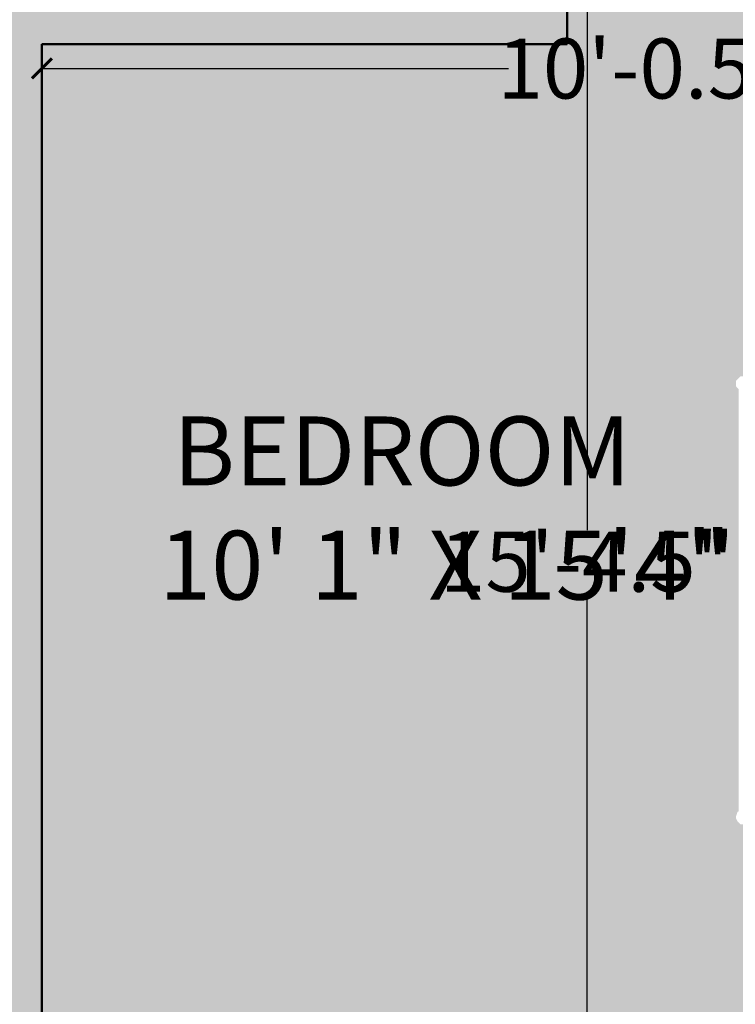
# Model space of a CAD drawing. Units: inches. Extents: x 528 to 2620, y -1066 to 798.
# Tile 12 of 41: x 776 to 848, y 573 to 672. Entities that reach past the tile are written whole.
import ezdxf

# ---------------------------------------------------------------- set-up
doc = ezdxf.new("R2010")
doc.units = ezdxf.units.IN
doc.header["$MEASUREMENT"] = 0
for name, color, linetype, lineweight in [('A-ANNO-DIMS', 2, 'Continuous', 18), ('A-AREA-IDEN', 7, 'Continuous', 18), ('A-WALL', 7, 'Continuous', 50), ('A-WALL-PATT', 8, 'Continuous', 13)]:
    doc.layers.add(name, color=color, linetype=linetype, lineweight=lineweight)
doc.styles.get("Standard").update_dxf_attribs({"font": 'arial.ttf'})
doc.dimstyles.get("Standard").update_dxf_attribs({"dimtxt": 6, "dimasz": 2, "dimexe": 0.18, "dimexo": 0.0625, "dimgap": 0.09, "dimtad": 0, "dimtih": 1, "dimtoh": 1, "dimdec": 1, "dimzin": 0, "dimdsep": 46, "dimlunit": 3, "dimtxsty": 'Standard', "dimblk": 'ARCHTICK', "dimcen": 0.09, "dimadec": 0, "dimazin": 0, "dimtfac": 1, "dimtdec": 1, "dimtofl": 0, "dimtmove": 0, "dimatfit": 3, "dimfxl": 1, "dimtolj": 1, "dimtzin": 0, "dimarcsym": 0})

# ---------------------------------------------------------------- blocks, each defined once
blk = doc.blocks.new('_ArchTick')
at = {"color": 0, "linetype": 'ByBlock', "const_width": 0.15}
blk.add_lwpolyline([(-0.5, -0.5), (0.5, 0.5)], dxfattribs=at)
blk = doc.blocks.new('*D27')
at = {"layer": 'A-ANNO-DIMS', "color": 0, "lineweight": -2, "transparency": 16777216}
for p, q in [((778.559, 667.76), (778.559, 666.811)), ((899.059, 667.76), (899.059, 666.811)), ((778.559, 666.991), (825.201, 666.991)), ((899.059, 666.991), (852.418, 666.991))]:
    blk.add_line(p, q, dxfattribs=at)
at = {"layer": 'Defpoints', "color": 0, "transparency": 16777216}
for p in [(778.559, 667.823), (899.059, 667.823), (899.059, 666.991)]:
    blk.add_point(p, dxfattribs=at)
at = {"layer": 'A-ANNO-DIMS', "color": 0, "lineweight": -2, "transparency": 16777216, "xscale": 2, "yscale": 2, "zscale": 2, "rotation": 180}
blk.add_blockref('_ArchTick', (778.559, 666.991), dxfattribs=at)
at = {"layer": 'A-ANNO-DIMS', "color": 0, "lineweight": -2, "transparency": 16777216, "xscale": 2, "yscale": 2, "zscale": 2}
blk.add_blockref('_ArchTick', (899.059, 666.991), dxfattribs=at)
at = {"layer": 'A-ANNO-DIMS', "color": 0, "transparency": 16777216, "insert": (838.809, 666.991), "char_height": 6, "attachment_point": 5}
blk.add_mtext('\\A1;10\'-0.5"', dxfattribs=at)
blk = doc.blocks.new('*D28')
at = {"layer": 'A-ANNO-DIMS', "color": 0, "lineweight": -2, "transparency": 16777216}
for p, q in [((833.059, 709.922), (833.059, 620.826)), ((833.122, 709.922), (833.239, 709.922)), ((833.059, 525.422), (833.059, 614.519)), ((833.102, 525.422), (832.879, 525.422))]:
    blk.add_line(p, q, dxfattribs=at)
at = {"layer": 'Defpoints', "color": 0, "transparency": 16777216}
for p in [(833.059, 709.922), (833.059, 709.922), (833.164, 525.422)]:
    blk.add_point(p, dxfattribs=at)
at = {"layer": 'A-ANNO-DIMS', "color": 0, "lineweight": -2, "transparency": 16777216, "xscale": 2, "yscale": 2, "zscale": 2}
for p, rotation in [((833.059, 709.922), 90), ((833.059, 525.422), 270)]:
    blk.add_blockref('_ArchTick', p, dxfattribs=dict(at, rotation=rotation))
at = {"layer": 'A-ANNO-DIMS', "color": 0, "transparency": 16777216, "insert": (833.059, 617.672), "char_height": 6, "attachment_point": 5}
blk.add_mtext('\\A1;15\'-4.5"', dxfattribs=at)

msp = doc.modelspace()

# ---------------------------------------------------------------- hatches: boundary and pattern name
at = {"layer": 'A-WALL-PATT', "transparency": 33554687}
h = msp.add_hatch(color=256, dxfattribs=at)
h.dxf.hatch_style = 1
h.paths.add_polyline_path([(861.059, 273.922), (817.059, 273.922), (817.059, 272.922), (861.059, 272.922)])
h.paths.add_polyline_path([(817.059, 277.922), (815.059, 277.922), (815.059, 268.922), (817.059, 268.922)])
h.paths.add_polyline_path([(908.059, 397.922), (899.059, 397.922), (899.059, 395.922), (908.059, 395.922)])
h.paths.add_polyline_path([(908.059, 443.922), (899.059, 443.922), (899.059, 441.922), (908.059, 441.922)])
h.paths.add_polyline_path([(904.059, 441.922), (903.059, 441.922), (903.059, 397.922), (904.059, 397.922)])
h.paths.add_polyline_path([(625.059, 561.422), (624.059, 561.422), (624.059, 537.422), (625.059, 537.422)])
h.paths.add_polyline_path([(648.747, 334.444), (720.045, 334.444), (720.045, 344.998), (648.747, 344.998)], flags=9)
h.paths.add_polyline_path([(819.733, 323.153), (880.328, 323.153), (880.328, 333.708), (819.733, 333.708)], flags=9)
h.paths.add_polyline_path([(779.898, 680.607), (821.764, 680.607), (821.764, 691.169), (779.898, 691.169)], flags=9)
h.paths.add_polyline_path([(779.876, 692.362), (817.138, 692.362), (817.138, 703.058), (779.876, 703.058)], flags=9)
h.paths.add_polyline_path([(799.994, 453.884), (860.589, 453.884), (860.589, 464.439), (799.994, 464.439)], flags=9)
h.paths.add_polyline_path([(650.866, 539.397), (708.781, 539.397), (708.781, 549.952), (650.866, 549.952)], flags=9)
h.paths.add_polyline_path([(788.504, 612.01), (849.099, 612.01), (849.099, 622.565), (788.504, 622.565)], flags=9)
h.paths.add_polyline_path([(639.539, 648.31), (700.134, 648.31), (700.134, 658.865), (639.539, 658.865)], flags=9)
h.paths.add_polyline_path([(648.913, 346.09), (747.706, 346.09), (747.706, 356.778), (648.913, 356.778)], flags=9)
h.paths.add_polyline_path([(676.857, 450.66), (746.735, 450.66), (746.735, 461.355), (676.857, 461.355)], flags=9)
h.paths.add_polyline_path([(819.711, 334.947), (865.526, 334.947), (865.526, 345.636), (819.711, 345.636)], flags=9)
h.paths.add_polyline_path([(806.298, 467.745), (874.047, 467.745), (874.047, 478.441), (806.298, 478.441)], flags=9)
h.paths.add_polyline_path([(653.235, 552.284), (690.497, 552.284), (690.497, 562.979), (653.235, 562.979)], flags=9)
h.paths.add_polyline_path([(789.903, 623.407), (843.208, 623.407), (843.208, 634.103), (789.903, 634.103)], flags=9)
h.paths.add_polyline_path([(639.773, 662.103), (693.077, 662.103), (693.077, 672.798), (639.773, 672.798)], flags=9)
h.paths.add_polyline_path([(801.587, 242.914), (846.334, 242.914), (846.334, 253.603), (801.587, 253.603)], flags=9)
h.paths.add_polyline_path([(925.362, 593.982), (925.362, 674.057), (914.673, 674.057), (914.673, 593.982)], flags=9)
h.paths.add_polyline_path([(612.559, 593.982), (612.559, 674.057), (601.871, 674.057), (601.871, 593.982)], flags=9)
h.paths.add_polyline_path([(723.31, 726.564), (803.385, 726.564), (803.385, 737.252), (723.31, 737.252)], flags=9)
at = {"layer": 'A-WALL-PATT', "transparency": 33554521}
h = msp.add_hatch(color=256, dxfattribs=at)
h.dxf.hatch_style = 1
h.paths.add_polyline_path([(629.059, 709.922), (677.559, 709.922), (677.559, 718.922), (620.059, 718.922), (620.059, 667.922), (629.059, 667.922)])
h.paths.add_polyline_path([(790.559, 718.922), (725.559, 718.922), (725.559, 709.922), (774.059, 709.922), (774.059, 577.922), (768.481, 577.922), (768.559, 573.422), (774.059, 573.422), (774.059, 567.422), (778.559, 567.422), (778.559, 669.422), (831.059, 669.422), (831.059, 675.922), (826.559, 675.922), (826.559, 673.922), (778.559, 673.922), (778.559, 709.922), (790.559, 709.922)])
h.paths.add_polyline_path([(908.059, 718.922), (879.059, 718.922), (879.059, 709.922), (899.059, 709.922), (899.059, 641.672), (908.059, 641.672)])
h.paths.add_polyline_path([(629.059, 619.922), (620.059, 619.922), (620.059, 561.422), (629.059, 561.422), (629.059, 573.422), (724.059, 573.422), (724.059, 569.422), (728.559, 569.422), (728.559, 577.922), (629.059, 577.922)])
h.paths.add_polyline_path([(779.059, 391.422), (779.059, 400.422), (770.059, 400.422), (764.059, 400.422), (764.059, 397.422), (764.059, 391.422), (770.059, 391.422), (770.059, 268.922), (815.059, 268.922), (815.059, 277.922), (779.059, 277.922), (779.059, 359.767)])
h.paths.add_polyline_path([(908.059, 395.922), (899.059, 395.922), (851.059, 395.922), (851.059, 391.422), (899.059, 391.422), (899.059, 277.922), (863.059, 277.922), (863.059, 268.922), (908.059, 268.922)])
h.paths.add_polyline_path([(908.059, 593.672), (899.059, 593.672), (899.059, 525.422), (778.559, 525.422), (778.559, 527.172), (774.059, 527.172), (774.059, 520.922), (899.059, 520.922), (899.059, 443.922), (908.059, 443.922)])
h.paths.add_polyline_path([(629.059, 520.922), (728.559, 520.922), (728.559, 545.422), (724.059, 545.422), (724.059, 525.422), (629.059, 525.422), (629.059, 537.422), (620.059, 537.422), (620.059, 484.672), (629.059, 484.672)])
h.paths.add_polyline_path([(629.059, 436.672), (620.059, 436.672), (620.059, 391.422), (648.559, 391.422), (648.559, 400.422), (629.059, 400.422)])
h.paths.add_polyline_path([(716.059, 397.422), (716.059, 400.422), (696.559, 400.422), (696.559, 391.422), (716.059, 391.422)])
at = {"layer": 'A-WALL-PATT', "transparency": 33554590}
h = msp.add_hatch(color=256, dxfattribs=at)
h.dxf.hatch_style = 1
h.paths.add_polyline_path([(774.059, 709.922), (629.059, 709.922), (629.059, 577.922), (728.559, 577.922), (728.559, 579.422), (728.559, 619.422), (730.309, 619.422), (730.309, 619.384, -0.401453), (768.559, 579.422), (768.559, 577.922), (774.059, 577.922)])
h.paths.add_polyline_path([(723.896, 686.058), (723.968, 686.064), (723.828, 686.128)], flags=0)
h.paths.add_polyline_path([(722.785, 642.699), (722.893, 642.756), (722.893, 684.992), (722.647, 685.244), (722.647, 685.82), (723.079, 686.262), (723.533, 686.262), (723.968, 686.064), (724.739, 686.128), (770.696, 686.128), (770.78, 686.14), (771.126, 686.266), (771.694, 686.094), (771.94, 685.478), (771.67, 684.904), (771.582, 684.871), (771.582, 642.782), (771.878, 642.514), (771.878, 641.921), (771.511, 641.462), (770.855, 641.462), (770.401, 641.833), (770.401, 641.551), (724.739, 641.551), (723.991, 641.705), (723.443, 641.414), (722.879, 641.585), (722.597, 642.142)], flags=16)
h.paths.add_polyline_path([(723.994, 641.704), (723.994, 641.707), (723.991, 641.705)], flags=0)
h.paths.add_polyline_path([(722.893, 642.732), (722.893, 684.992), (722.647, 685.244), (722.647, 685.82), (723.079, 686.262), (723.287, 686.262), (722.991, 686.172), (722.794, 685.971), (722.647, 685.68), (722.647, 685.434), (722.745, 685.143), (722.942, 684.942), (723.238, 684.807), (723.484, 684.807), (723.779, 684.897), (723.976, 685.098), (724.174, 685.488), (724.124, 685.635), (724.124, 685.249), (723.631, 684.746), (723.631, 642.961), (724.124, 642.514), (724.124, 641.887), (723.656, 641.462), (723.079, 641.462), (722.647, 641.904), (722.647, 642.48)], flags=0)
h.paths.add_polyline_path([(722.647, 642.29), (722.647, 642.044), (722.794, 641.753), (723.079, 641.462), (723.287, 641.462), (722.879, 641.585), (722.597, 642.142)], flags=0)
h.paths.add_polyline_path([(770.745, 686.128), (770.58, 686.128), (770.551, 686.057)], flags=0)
h.paths.add_polyline_path([(743.299, 645.288), (753.227, 659.398), (748.69, 663.75), (753.234, 668.538), (743.299, 682.458), (743.791, 682.592), (744.136, 682.681), (744.53, 682.928), (744.628, 683.084), (745.017, 683.327), (744.53, 684.069), (744.776, 684.158), (744.874, 684.315), (745.514, 684.404), (746.081, 684.651), (746.474, 684.651), (746.819, 684.807), (747.459, 685.031), (747.705, 685.143), (748.198, 685.277), (748.394, 685.523), (748.862, 685.523), (749.994, 686.128), (753.488, 676.03), (757.379, 680.153), (757.791, 679.758), (758.044, 680.645), (758.29, 681.227), (758.29, 682.055), (758.019, 682.592), (757.871, 683.174), (757.822, 683.778), (758.388, 684.069), (758.979, 684.203), (759.619, 684.158), (760.21, 683.957), (760.751, 683.666), (761.859, 683.666), (762.401, 683.957), (762.991, 684.114), (763.631, 684.114), (764.198, 683.957), (764.739, 683.666), (766.118, 683.666), (766.659, 683.957), (767.25, 684.158), (767.865, 684.203), (768.456, 684.069), (769.047, 683.778), (768.998, 683.174), (768.85, 682.592), (768.554, 682.055), (768.554, 681.227), (768.801, 680.645), (769.092, 679.75), (768.948, 678.832), (768.801, 678.228), (768.554, 677.646), (768.554, 676.818), (768.801, 676.237), (769.092, 675.341), (768.948, 674.424), (768.801, 673.82), (768.554, 673.283), (768.554, 672.41), (768.801, 671.873), (768.998, 671.291), (769.047, 670.642), (768.948, 670.016), (768.801, 669.411), (768.554, 668.874), (768.554, 668.002), (768.974, 667.239), (769.047, 666.279), (769.047, 665.563), (768.456, 665.316), (767.865, 665.16), (767.25, 665.16), (766.659, 665.361), (766.118, 665.697), (764.739, 665.697), (763.945, 665.204), (762.991, 665.204), (762.401, 665.361), (761.859, 665.697), (761.005, 665.697), (762.696, 664.086), (760.741, 662.027), (761.859, 662.027), (762.401, 662.318), (763.342, 662.548), (764.247, 662.318), (764.788, 662.027), (766.118, 662.027), (766.659, 662.318), (767.25, 662.519), (767.865, 662.564), (768.505, 662.43), (769.047, 662.116), (769.047, 661.4), (769.047, 660.796), (768.85, 660.214), (768.554, 659.677), (768.554, 658.849), (768.85, 658.267), (768.998, 657.663), (769.069, 656.749), (768.85, 655.851), (768.554, 655.269), (768.554, 654.441), (768.85, 653.859), (769.069, 652.961), (768.998, 652.046), (768.85, 651.442), (768.554, 650.905), (768.554, 650.032), (768.85, 649.495), (768.998, 648.914), (769.047, 648.265), (768.998, 647.638), (768.85, 647.034), (768.554, 646.497), (768.554, 645.624), (768.85, 645.087), (769.047, 644.55), (769.047, 643.901), (768.505, 643.655), (767.865, 643.521), (767.25, 643.521), (766.659, 643.722), (766.118, 644.058), (764.788, 644.058), (764.247, 643.722), (763.342, 643.492), (762.401, 643.722), (761.859, 644.058), (760.801, 644.058), (760.259, 643.722), (759.668, 643.521), (759.028, 643.521), (758.388, 643.655), (757.871, 643.901), (757.871, 644.55), (758.044, 645.087), (758.339, 645.624), (758.339, 646.497), (758.044, 647.034), (757.921, 647.638), (757.866, 648.059), (757.379, 647.593), (753.422, 651.773), (749.994, 641.618), (749.502, 641.708), (749.354, 641.954), (748.542, 642.446), (747.311, 642.939), (746.652, 642.939), (746.327, 643.185), (745.514, 643.565), (744.53, 643.655), (745.011, 644.4), (744.628, 644.639), (744.136, 644.886), (743.791, 645.132)], flags=0)
h.paths.add_polyline_path([(755.656, 654.933), (756.542, 654.687), (757.527, 654.329), (756.641, 654.575)], flags=0)
h.paths.add_polyline_path([(758.339, 649.204), (758.339, 648.712), (758.585, 644.304), (758.585, 648.802)], flags=0)
h.paths.add_polyline_path([(758.339, 649.294), (758.093, 649.697), (758.359, 649.165)], flags=0)
h.paths.add_polyline_path([(755.656, 672.79), (756.493, 673.037), (757.358, 673.351), (757.353, 673.358), (756.641, 673.149)], flags=0)
h.paths.add_polyline_path([(760.264, 639.641), (771.408, 639.641), (771.408, 624.039), (760.264, 624.039)], flags=16)
h.paths.add_polyline_path([(761.378, 638.526), (770.294, 638.526), (770.294, 625.153), (761.378, 625.153)], flags=0)
edge = h.paths.add_edge_path(flags=0)
edge.add_ellipse((765.836, 631.84), major_axis=(-2.245, 2.245), ratio=1, start_angle=-45, end_angle=45, ccw=False)
edge.add_ellipse((765.836, 631.84), major_axis=(-2.245, 2.245), ratio=1, start_angle=-135, end_angle=-45, ccw=False)
edge.add_ellipse((765.836, 631.84), major_axis=(-2.245, 2.245), ratio=1, start_angle=135, end_angle=-135, ccw=False)
edge.add_ellipse((765.836, 631.84), major_axis=(-2.245, 2.245), ratio=1, start_angle=45, end_angle=135, ccw=False)
h.paths.add_polyline_path([(758.585, 683.42), (758.585, 678.922), (758.373, 678.575), (758.339, 678.43), (758.093, 678.049), (758.339, 678.519), (758.339, 679.011)], flags=0)
h.paths.add_polyline_path([(760.264, 688.038), (760.264, 703.64), (771.408, 703.64), (771.408, 688.038)], flags=16)
h.paths.add_polyline_path([(770.401, 685.389), (770.401, 685.846), (770.855, 686.217), (771.511, 686.217), (771.878, 685.758), (771.878, 685.165), (771.582, 684.897), (771.582, 642.782), (771.878, 642.514), (771.878, 641.921), (771.511, 641.462), (770.855, 641.462), (770.401, 641.833), (770.401, 642.29)], flags=0)
h.paths.add_polyline_path([(770.532, 642.678), (771.052, 643.009), (771.67, 642.775), (771.94, 642.201), (771.694, 641.585), (771.126, 641.413), (770.551, 641.622), (770.347, 642.132)], flags=16)
h.paths.add_polyline_path([(761.378, 689.152), (761.378, 702.526), (770.294, 702.526), (770.294, 689.152)], flags=0)
edge = h.paths.add_edge_path(flags=0)
edge.add_ellipse((765.836, 695.839), major_axis=(2.245, 2.245), ratio=1, start_angle=405, end_angle=495, ccw=False)
edge.add_ellipse((765.836, 695.839), major_axis=(2.245, 2.245), ratio=1, start_angle=675, end_angle=765, ccw=False)
edge.add_ellipse((765.836, 695.839), major_axis=(2.245, 2.245), ratio=1, start_angle=585, end_angle=675, ccw=False)
edge.add_ellipse((765.836, 695.839), major_axis=(2.245, 2.245), ratio=1, start_angle=495, end_angle=585, ccw=False)
h.paths.add_polyline_path([(770.696, 684.897), (770.942, 684.74), (771.41, 684.74), (771.73, 685.031), (771.878, 685.344), (771.878, 685.635), (771.694, 686.094), (771.582, 686.128), (771.878, 685.758), (771.878, 685.165), (771.41, 684.74), (770.849, 684.74)], flags=0)
h.paths.add_polyline_path([(899.059, 709.922), (831.059, 709.922), (831.059, 699.922), (829.809, 699.922), (829.809, 675.922), (831.059, 675.922), (831.059, 669.422), (778.559, 669.422), (778.559, 567.172), (780.059, 567.172), (820.059, 567.172), (820.059, 565.422), (820.021, 565.422, -0.401453), (780.059, 527.172), (778.559, 527.172), (778.559, 525.422), (899.059, 525.422)])
h.paths.add_polyline_path([(849.197, 636.014), (849.269, 636.02), (849.129, 636.084)], flags=0)
h.paths.add_polyline_path([(848.193, 634.948), (847.947, 635.2), (847.947, 635.776), (848.379, 636.218), (848.833, 636.218), (849.269, 636.02), (850.039, 636.084), (895.996, 636.084), (896.081, 636.096), (896.426, 636.222), (896.995, 636.05), (897.241, 635.434), (896.97, 634.86), (896.883, 634.827), (896.883, 592.738), (897.178, 592.47), (897.178, 591.877), (896.811, 591.418), (896.155, 591.418), (895.701, 591.789), (895.701, 591.507), (850.039, 591.507), (849.292, 591.661), (848.744, 591.37), (848.18, 591.541), (847.897, 592.098), (848.086, 592.655), (848.193, 592.712)], flags=16)
h.paths.add_polyline_path([(849.294, 591.66), (849.295, 591.663), (849.292, 591.661)], flags=16)
h.paths.add_polyline_path([(848.193, 634.948), (847.947, 635.2), (847.947, 635.776), (848.379, 636.218), (848.587, 636.218), (848.292, 636.128), (848.095, 635.927), (847.947, 635.636), (847.947, 635.39), (848.046, 635.099), (848.243, 634.897), (848.538, 634.763), (848.784, 634.763), (849.079, 634.853), (849.276, 635.054), (849.474, 635.444), (849.424, 635.591), (849.424, 635.205), (848.932, 634.702), (848.932, 592.917), (849.424, 592.47), (849.424, 591.843), (848.956, 591.418), (848.379, 591.418), (847.947, 591.86), (847.947, 592.436), (848.193, 592.688)], flags=0)
h.paths.add_polyline_path([(847.947, 592.246), (847.947, 592), (848.095, 591.709), (848.379, 591.418), (848.587, 591.418), (848.18, 591.541), (847.897, 592.098)], flags=16)
h.paths.add_polyline_path([(896.046, 636.084), (895.88, 636.084), (895.852, 636.013)], flags=0)
h.paths.add_polyline_path([(868.599, 632.414), (869.092, 632.548), (869.436, 632.637), (869.83, 632.884), (869.929, 633.04), (870.318, 633.283), (869.83, 634.025), (870.076, 634.114), (870.175, 634.271), (870.815, 634.36), (871.381, 634.607), (871.775, 634.607), (872.119, 634.763), (872.759, 634.987), (873.006, 635.099), (873.498, 635.233), (873.695, 635.479), (874.163, 635.479), (875.295, 636.084), (878.788, 625.986), (882.679, 630.109), (883.091, 629.714), (883.344, 630.601), (883.59, 631.183), (883.59, 632.011), (883.319, 632.548), (883.172, 633.13), (883.123, 633.734), (883.689, 634.025), (884.279, 634.159), (884.919, 634.114), (885.51, 633.913), (886.052, 633.622), (887.159, 633.622), (887.701, 633.913), (888.292, 634.07), (888.932, 634.07), (889.498, 633.913), (890.039, 633.622), (891.418, 633.622), (891.959, 633.913), (892.55, 634.114), (893.166, 634.159), (893.756, 634.025), (894.347, 633.734), (894.298, 633.13), (894.15, 632.548), (893.855, 632.011), (893.855, 631.183), (894.101, 630.601), (894.393, 629.706), (894.249, 628.788), (894.101, 628.184), (893.855, 627.602), (893.855, 626.774), (894.101, 626.193), (894.393, 625.297), (894.249, 624.38), (894.101, 623.776), (893.855, 623.239), (893.855, 622.366), (894.101, 621.829), (894.298, 621.247), (894.347, 620.598), (894.249, 619.972), (894.101, 619.367), (893.855, 618.83), (893.855, 617.958), (894.274, 617.195), (894.347, 616.235), (894.347, 615.518), (893.756, 615.272), (893.166, 615.116), (892.55, 615.116), (891.959, 615.317), (891.418, 615.653), (890.039, 615.653), (889.245, 615.16), (888.292, 615.16), (887.701, 615.317), (887.159, 615.653), (886.305, 615.653), (887.996, 614.042), (886.041, 611.983), (887.159, 611.983), (887.701, 612.274), (888.642, 612.504), (889.547, 612.274), (890.089, 611.983), (891.418, 611.983), (891.959, 612.274), (892.55, 612.475), (893.166, 612.52), (893.806, 612.386), (894.347, 612.072), (894.347, 611.356), (894.347, 610.752), (894.15, 610.17), (893.855, 609.633), (893.855, 608.805), (894.15, 608.223), (894.298, 607.619), (894.37, 606.705), (894.15, 605.807), (893.855, 605.225), (893.855, 604.397), (894.15, 603.815), (894.37, 602.917), (894.298, 602.002), (894.15, 601.398), (893.855, 600.861), (893.855, 599.988), (894.15, 599.451), (894.298, 598.87), (894.347, 598.221), (894.298, 597.594), (894.15, 596.99), (893.855, 596.453), (893.855, 595.58), (894.15, 595.043), (894.347, 594.506), (894.347, 593.857), (893.806, 593.611), (893.166, 593.477), (892.55, 593.477), (891.959, 593.678), (891.418, 594.014), (890.089, 594.014), (889.547, 593.678), (888.642, 593.448), (887.701, 593.678), (887.159, 594.014), (886.101, 594.014), (885.559, 593.678), (884.969, 593.477), (884.329, 593.477), (883.689, 593.611), (883.172, 593.857), (883.172, 594.506), (883.344, 595.043), (883.639, 595.58), (883.639, 596.453), (883.344, 596.99), (883.221, 597.594), (883.167, 598.015), (882.679, 597.549), (878.722, 601.729), (875.295, 591.574), (874.803, 591.664), (874.655, 591.91), (873.843, 592.402), (872.612, 592.895), (871.952, 592.895), (871.627, 593.141), (870.815, 593.521), (869.83, 593.611), (870.311, 594.356), (869.929, 594.595), (869.436, 594.842), (869.092, 595.088), (868.599, 595.244), (878.528, 609.354), (873.99, 613.706), (878.535, 618.494)], flags=0)
h.paths.add_polyline_path([(880.956, 622.746), (881.793, 622.993), (882.659, 623.307), (882.654, 623.314), (881.941, 623.104)], flags=0)
h.paths.add_polyline_path([(880.956, 604.889), (881.843, 604.643), (882.827, 604.285), (881.941, 604.531)], flags=16)
h.paths.add_polyline_path([(883.393, 628.005), (883.639, 628.475), (883.639, 628.967), (883.886, 633.376), (883.886, 628.878), (883.674, 628.531), (883.639, 628.386)], flags=0)
h.paths.add_polyline_path([(883.639, 599.16), (883.639, 598.668), (883.886, 594.26), (883.886, 598.758)], flags=16)
h.paths.add_polyline_path([(883.639, 599.25), (883.393, 599.653), (883.659, 599.121)], flags=16)
h.paths.add_polyline_path([(885.564, 637.994), (885.564, 653.596), (896.709, 653.596), (896.709, 637.994)], flags=16)
h.paths.add_polyline_path([(885.564, 589.597), (896.709, 589.597), (896.709, 573.995), (885.564, 573.995)], flags=16)
h.paths.add_polyline_path([(886.679, 639.108), (886.679, 652.482), (895.594, 652.482), (895.594, 639.108)], flags=0)
h.paths.add_polyline_path([(886.679, 588.482), (895.594, 588.482), (895.594, 575.109), (886.679, 575.109)], flags=0)
edge = h.paths.add_edge_path(flags=0)
edge.add_ellipse((891.136, 645.795), major_axis=(2.245, 2.245), ratio=1, start_angle=405, end_angle=495, ccw=False)
edge.add_ellipse((891.136, 645.795), major_axis=(2.245, 2.245), ratio=1, start_angle=675, end_angle=765, ccw=False)
edge.add_ellipse((891.136, 645.795), major_axis=(2.245, 2.245), ratio=1, start_angle=585, end_angle=675, ccw=False)
edge.add_ellipse((891.136, 645.795), major_axis=(2.245, 2.245), ratio=1, start_angle=495, end_angle=585, ccw=False)
edge = h.paths.add_edge_path(flags=0)
edge.add_ellipse((891.136, 581.796), major_axis=(-2.245, 2.245), ratio=1, start_angle=-45, end_angle=45, ccw=False)
edge.add_ellipse((891.136, 581.796), major_axis=(-2.245, 2.245), ratio=1, start_angle=-135, end_angle=-45, ccw=False)
edge.add_ellipse((891.136, 581.796), major_axis=(-2.245, 2.245), ratio=1, start_angle=135, end_angle=-135, ccw=False)
edge.add_ellipse((891.136, 581.796), major_axis=(-2.245, 2.245), ratio=1, start_angle=45, end_angle=135, ccw=False)
h.paths.add_polyline_path([(895.701, 635.345), (895.701, 635.802), (896.155, 636.173), (896.811, 636.173), (897.178, 635.714), (897.178, 635.121), (896.883, 634.853), (896.883, 592.738), (897.178, 592.47), (897.178, 591.877), (896.811, 591.418), (896.155, 591.418), (895.701, 591.789), (895.701, 592.246)], flags=0)
h.paths.add_polyline_path([(895.996, 634.853), (896.243, 634.696), (896.71, 634.696), (897.03, 634.987), (897.178, 635.3), (897.178, 635.591), (896.995, 636.05), (896.883, 636.084), (897.178, 635.714), (897.178, 635.121), (896.71, 634.696), (896.15, 634.696)], flags=0)
h.paths.add_polyline_path([(895.832, 592.634), (896.353, 592.965), (896.97, 592.731), (897.241, 592.157), (896.995, 591.541), (896.426, 591.369), (895.852, 591.578), (895.648, 592.088)], flags=16)
h.paths.add_polyline_path([(725.255, 569.422), (724.059, 569.422), (724.059, 573.422), (629.059, 573.422), (629.059, 525.422), (724.059, 525.422), (724.059, 545.422), (725.255, 545.422)])
h.paths.add_polyline_path([(820.021, 565.422), (780.059, 565.422), (780.059, 567.172), (774.059, 567.172), (774.059, 567.422), (774.059, 573.422), (768.559, 573.422), (768.481, 577.922), (768.559, 577.922), (768.559, 579.422, 0.401453), (730.309, 619.384), (730.309, 579.422), (728.559, 579.422), (728.559, 573.422), (728.559, 569.422), (727.255, 569.422), (727.255, 545.422), (728.559, 545.422), (728.559, 520.922), (665.059, 520.922), (665.059, 436.422), (716.059, 436.422), (716.059, 421.422), (717.809, 421.422), (717.809, 421.358, -0.392996), (740.059, 397.422, -0.392996), (762.309, 421.358), (762.309, 421.422), (764.059, 421.422), (764.059, 400.422), (770.059, 400.422), (779.059, 400.422), (779.059, 391.422), (779.059, 359.767), (795.432, 359.767), (795.432, 294.295), (893.669, 294.295), (893.669, 277.922), (899.059, 277.922), (899.059, 391.422), (851.059, 391.422), (851.059, 395.922), (899.059, 395.922), (899.059, 443.922), (899.059, 520.922), (774.059, 520.922), (774.059, 527.172), (778.559, 527.172), (780.059, 527.172, 0.401453)])
h.paths.add_polyline_path([(774.059, 519.657), (842.122, 519.657), (842.122, 505.072), (788.644, 505.072), (788.644, 474.079), (788.644, 470.433, -0.883215), (779.529, 456.663), (774.971, 456.663, -0.414214), (774.059, 457.575)], flags=16)
h.paths.add_polyline_path([(775.883, 517.834), (840.299, 517.834), (840.299, 514.188), (788.644, 514.188), (788.644, 484.41), (779.529, 484.41), (779.529, 474.079), (775.883, 474.079)], flags=0)
h.paths.add_polyline_path([(706.7, 501.564, -0.254069), (706.7, 493.021), (698.31, 492.555), (698.31, 502.031)], flags=16)
h.paths.add_polyline_path([(691.334, 515.692), (691.8, 507.301), (682.325, 507.301), (682.791, 515.692, -0.254069)], flags=16)
h.paths.add_polyline_path([(695.485, 504.685), (695.485, 479.416), (678.64, 479.416), (678.64, 504.685)], flags=16)
h.paths.add_polyline_path([(706.7, 489.602, -0.254069), (706.7, 481.058), (698.31, 480.592), (698.31, 490.068)], flags=16)
h.paths.add_polyline_path([(675.815, 502.031), (675.815, 492.555), (667.425, 493.021, -0.254069), (667.425, 501.564)], flags=16)
h.paths.add_polyline_path([(691.8, 476.8), (691.334, 468.409, -0.254069), (682.791, 468.409), (682.325, 476.8)], flags=16)
h.paths.add_polyline_path([(675.815, 490.068), (675.815, 480.592), (667.425, 481.058, -0.254069), (667.425, 489.602)], flags=16)
h.paths.add_polyline_path([(764.059, 397.422), (762.309, 397.422), (762.309, 421.358, 0.392996), (740.059, 397.422, 0.392996), (717.809, 421.358), (717.809, 397.422), (716.059, 397.422), (716.059, 391.422), (716.059, 385.422), (764.059, 385.422), (764.059, 391.422)], flags=17)
h.paths.add_polyline_path([(716.059, 436.422), (705.859, 436.422), (705.859, 418.422), (716.059, 418.422), (716.059, 421.422)], flags=17)
h.paths.add_polyline_path([(716.059, 418.422), (705.859, 418.422), (705.859, 400.422), (716.059, 400.422)], flags=17)
h.paths.add_polyline_path([(705.859, 418.422), (695.659, 418.422), (695.659, 400.422), (696.559, 400.422), (705.859, 400.422)], flags=17)
h.paths.add_polyline_path([(705.859, 436.422), (695.659, 436.422), (695.659, 418.422), (705.859, 418.422)], flags=17)
h.paths.add_polyline_path([(695.659, 418.422), (685.459, 418.422), (685.459, 400.422), (695.659, 400.422)], flags=17)
h.paths.add_polyline_path([(695.659, 436.422), (685.459, 436.422), (685.459, 418.422), (695.659, 418.422)], flags=17)
h.paths.add_polyline_path([(685.459, 418.422), (675.259, 418.422), (675.259, 400.422), (685.459, 400.422)], flags=17)
h.paths.add_polyline_path([(685.459, 436.422), (675.259, 436.422), (675.259, 418.422), (685.459, 418.422)], flags=17)
h.paths.add_polyline_path([(675.259, 436.422), (665.059, 436.422), (665.059, 418.422), (675.259, 418.422)])
h.paths.add_polyline_path([(675.259, 418.422), (665.059, 418.422), (665.059, 400.422), (675.259, 400.422)])
h.paths.add_polyline_path([(665.059, 418.422), (646.967, 418.422), (646.991, 436.422), (629.059, 436.422), (629.059, 400.422), (665.059, 400.422)])
h.paths.add_polyline_path([(665.059, 436.422), (646.991, 436.422), (646.967, 418.422), (665.059, 418.422)], flags=17)
h.paths.add_polyline_path([(647.005, 446.622), (629.059, 446.622), (629.059, 436.672), (629.059, 436.422), (646.991, 436.422)])
h.paths.add_polyline_path([(665.059, 446.622), (647.005, 446.622), (646.991, 436.422), (665.059, 436.422)])
h.paths.add_polyline_path([(647.019, 456.822), (629.059, 456.822), (629.059, 446.622), (647.005, 446.622)])
h.paths.add_polyline_path([(665.059, 456.822), (647.019, 456.822), (647.005, 446.622), (665.059, 446.622)])
h.paths.add_polyline_path([(647.032, 467.022), (629.059, 467.022), (629.059, 456.822), (647.019, 456.822)])
h.paths.add_polyline_path([(665.059, 467.022), (647.032, 467.022), (647.019, 456.822), (665.059, 456.822)])
h.paths.add_polyline_path([(665.059, 477.222), (647.046, 477.222), (647.032, 467.022), (665.059, 467.022)])
h.paths.add_polyline_path([(647.046, 477.222), (629.059, 477.222), (629.059, 467.022), (647.032, 467.022)])
h.paths.add_polyline_path([(647.059, 487.222), (629.059, 487.222), (629.059, 477.222), (647.046, 477.222), (647.048, 479.019), (645.53, 483.246), (640.877, 480.371)])
h.paths.add_polyline_path([(665.059, 520.922), (629.059, 520.922), (629.059, 487.222), (647.059, 487.222), (665.059, 487.222)])
h.paths.add_polyline_path([(665.059, 487.222), (647.059, 487.222), (653.224, 480.355), (648.578, 483.242), (647.048, 479.019), (647.046, 477.222), (665.059, 477.222)])

# ---------------------------------------------------------------- linework, layer by layer
at = {"layer": 'A-WALL'}
for p, q in [((831.059, 675.922), (831.059, 669.422)), ((831.059, 669.422), (778.559, 669.422)), ((778.559, 669.422), (778.559, 567.422))]:
    msp.add_line(p, q, dxfattribs=at)

# ---------------------------------------------------------------- texts
at = {"layer": 'A-AREA-IDEN'}
for s, height, p in [('BEDROOM', 6.8907, (791.686, 625.307)), ('10\' 1" X 15\'4"', 6.89074, (790.263, 613.887))]:
    msp.add_text(s, height=height, dxfattribs=at).set_placement(p)

# ---------------------------------------------------------------- dimensions: what is measured, and where the dimension line sits
at = {"layer": 'A-ANNO-DIMS'}
dim = msp.add_linear_dim(base=(833.059, 709.922), p1=(833.164, 525.422), p2=(833.059, 709.922), angle=90, dimstyle='Standard', override={"dimclrd": 0, "dimclre": 0, "dimclrt": 0}, dxfattribs=at)
dim.commit()
dim.dimension.update_dxf_attribs({"geometry": '*D28', "text_midpoint": (833.059, 617.672)})
dim = msp.add_linear_dim(base=(899.059, 666.991), p1=(778.559, 667.823), p2=(899.059, 667.823), dimstyle='Standard', override={"dimclrd": 0, "dimclre": 0, "dimclrt": 0}, dxfattribs=at)
dim.commit()
dim.dimension.update_dxf_attribs({"geometry": '*D27', "text_midpoint": (838.809, 666.991)})

doc.saveas('drawing.dxf')
